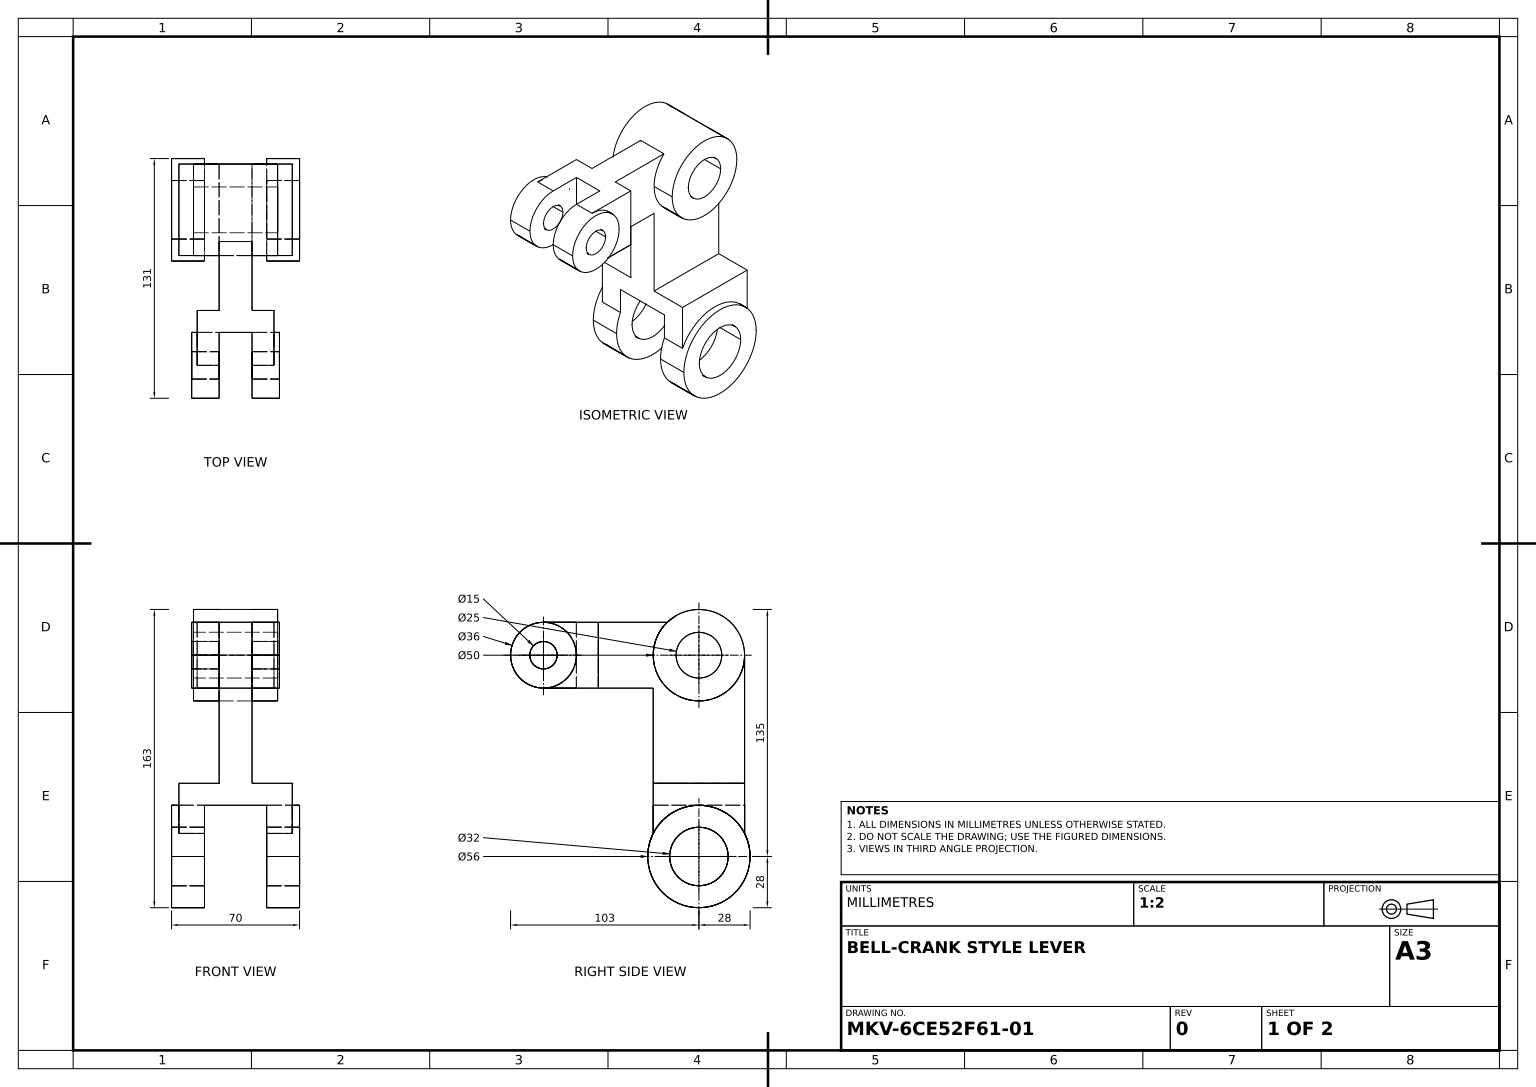
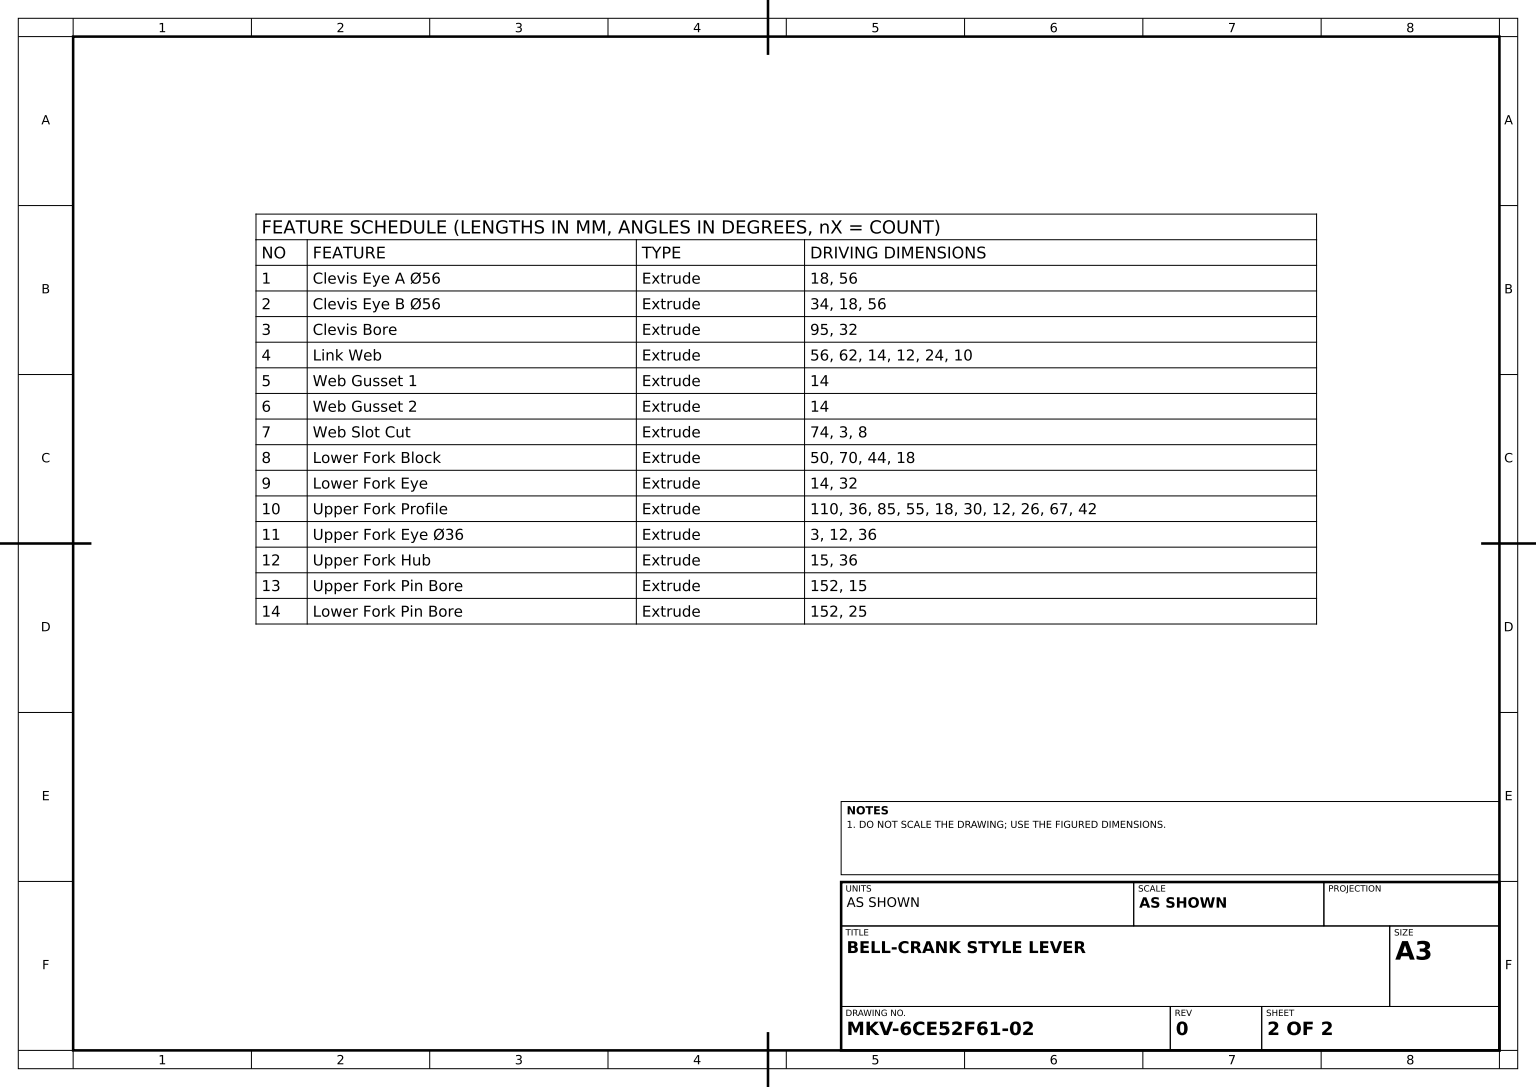
from build123d import *

# Parameters (mm, degrees)
CLEVIS_EYE_A_SKETCH_R        = 28
CLEVIS_EYE_A_56_DEPTH        = 18
CLEVIS_EYE_B_SKETCH_R        = 28
CLEVIS_EYE_B_56_DEPTH        = 18
CLEVIS_BORE_SKETCH_R         = 16
CLEVIS_BORE_DEPTH            = 95
LINK_WEB_DEPTH               = 28
WEB_GUSSET_1_DEPTH           = 14
WEB_START                    = -14
WEB_GUSSET_2_DEPTH           = 14
WEB_SLOT_CUT_DEPTH           = 74
LOWER_FORK_BLOCK_SKETCH_W    = 18
LOWER_FORK_BLOCK_SKETCH_H    = 70
LOWER_FORK_BLOCK_DEPTH       = 50
LOWER_FORK_EYE_DEPTH         = 14
LOWER_FORK_EYE_DEPTH_BACK    = 32
LOWER_FORK_EYE_SKETCH_R      = 25
UPPER_FORK_PROFILE_DEPTH     = 18
UPPER_FORK_EYE_36_DEPTH      = 3
UPPER_FORK_EYE_36_DEPTH_BACK = 12
UPPER_FORK_EYE_SKETCH_36_R   = 18
UPPER_FORK_HUB_SKETCH_R      = 18
UPPER_FORK_HUB_DEPTH         = 15
UPPER_FORK_PIN_BORE_SKETCH_R = 7.5
UPPER_FORK_PIN_BORE_DEPTH    = 152
LOWER_FORK_PIN_BORE_SKETCH_R = 12.5
LOWER_FORK_PIN_BORE_DEPTH    = 152


with BuildPart() as part:
    # Clevis Eye A Sketch → Clevis Eye A Ø56 (new body)
    with BuildSketch(Plane(origin=(0, 0, 0), x_dir=(0, 0, -1), z_dir=(1, 0, 0))):
        Circle(CLEVIS_EYE_A_SKETCH_R)
    extrude(amount=-CLEVIS_EYE_A_56_DEPTH)


with BuildPart() as body_2:
    # Clevis Eye B Sketch → Clevis Eye B Ø56 (new body)
    with BuildSketch(Plane.ZY.offset(52)):
        with Locations(Location((0, 0, 0), (0, 0, 180))):
            Circle(CLEVIS_EYE_B_SKETCH_R)
    extrude(amount=CLEVIS_EYE_B_56_DEPTH)


with BuildPart() as clevis_bore_tool:
    # Clevis Bore Sketch → Clevis Bore (new body)
    with BuildSketch(Plane(origin=(0, 0, 0), x_dir=(0, 0, -1), z_dir=(1, 0, 0))):
        Circle(CLEVIS_BORE_SKETCH_R)
    extrude(amount=-CLEVIS_BORE_DEPTH)


with BuildPart() as part_1:
    add(part.part)

    # Clevis Bore: cut by clevis_bore_tool
    add(clevis_bore_tool.part, mode=Mode.SUBTRACT)



with BuildPart() as body_2_1:
    add(body_2.part)

    # Clevis Bore: cut by clevis_bore_tool
    add(clevis_bore_tool.part, mode=Mode.SUBTRACT)


with BuildPart() as part_2:
    add(part_1.part)

    add(body_2_1.part)  # Link Web merges body 2
    # Link Web Sketch → Link Web (add, symmetric)
    with BuildSketch(Plane.XY):
        Polygon((-66, 40), (-66, 16), (-52, 16), (-52, 26), (-52, 28), (-18, 28), (-18, 26), (-18, 16), (-4, 16), (-4, 40), align=None)
    extrude(amount=LINK_WEB_DEPTH, both=True)

    # Web Gusset 1 Sketch → Web Gusset 1 (add)
    with BuildSketch(Plane(origin=(-4, 0, 0), x_dir=(0, 0, -1), z_dir=(1, 0, 0))):
        with BuildLine():
            Line((-28, 16), (-28, 0))
            ThreePointArc((-28, 0), (-26.71508, 8.384777), (-22.978251, 16))
            Line((-22.978251, 16), (-28, 16))
        make_face()
        with BuildLine():
            Line((28, 16), (28, 0))
            ThreePointArc((28, 0), (26.71508, 8.384777), (22.978251, 16))
            Line((22.978251, 16), (28, 16))
        make_face()
    extrude(amount=-WEB_GUSSET_1_DEPTH)

    # Web Gusset 2 Sketch → Web Gusset 2 (add)
    with BuildSketch(Plane.ZY.offset(66).offset(WEB_START)):
        with BuildLine():
            Line((28, 16), (28, 0))
            ThreePointArc((28, 0), (26.71508, 8.384777), (22.978251, 16))
            Line((22.978251, 16), (28, 16))
        make_face()
        with BuildLine():
            Line((-28, 0), (-28, 16))
            Line((-28, 16), (-22.978251, 16))
            ThreePointArc((-22.978251, 16), (-26.71508, 8.384777), (-28, 0))
        make_face()
    extrude(amount=WEB_GUSSET_2_DEPTH)

    # Web Slot Sketch → Web Slot Cut (cut)
    with BuildSketch(Plane(origin=(-4, 0, 0), x_dir=(0, 0, -1), z_dir=(1, 0, 0))):
        with BuildLine():
            Line((-25, 12.60952), (-25, 40))
            Line((-25, 40), (-28, 40))
            Line((-28, 40), (-28, 0))
            ThreePointArc((-28, 0), (-27.239677, 6.480741), (-25, 12.60952))
        make_face()
        with BuildLine():
            Line((28, 40), (25, 40))
            Line((25, 40), (25, 12.60952))
            ThreePointArc((25, 12.60952), (27.239677, 6.480741), (28, 0))
            Line((28, 0), (28, 40))
        make_face()
    extrude(amount=-WEB_SLOT_CUT_DEPTH, mode=Mode.SUBTRACT)

    # Lower Fork Block Sketch → Lower Fork Block (add)
    with BuildSketch(Plane.XY.offset(25)):
        with Locations((-35, 75)):
            Rectangle(LOWER_FORK_BLOCK_SKETCH_W, LOWER_FORK_BLOCK_SKETCH_H)
    extrude(amount=-LOWER_FORK_BLOCK_DEPTH)

    # Lower Fork Eye Sketch → Lower Fork Eye (add, two sides: drawn at the far end of the back side and taken through both)
    with BuildSketch(Plane.ZY.offset(44).offset(-LOWER_FORK_EYE_DEPTH_BACK)):
        with Locations((0, 110)):
            Circle(LOWER_FORK_EYE_SKETCH_R)
    extrude(amount=LOWER_FORK_EYE_DEPTH + LOWER_FORK_EYE_DEPTH_BACK)

    # Upper Fork Profile Sketch → Upper Fork Profile (add, symmetric)
    with BuildSketch(Plane(origin=(0, 110, 0), x_dir=(1, 0, 0), z_dir=(0, 1, 0))):
        Polygon((-26, -55), (-14, -55), (-14, -85), (-26, -85), (-26, -67), (-44, -67), (-44, -85), (-56, -85), (-56, -55), (-44, -55), (-44, 0), (-26, 0), align=None)
    extrude(amount=UPPER_FORK_PROFILE_DEPTH, both=True)

    # Upper Fork Eye Sketch Ø36 → Upper Fork Eye Ø36 (add, two sides: drawn at the far end of the back side and taken through both)
    with BuildSketch(Plane(origin=(-14, 0, 0), x_dir=(0, 0, -1), z_dir=(1, 0, 0)).offset(-UPPER_FORK_EYE_36_DEPTH_BACK)):
        with Locations((-85, 110)):
            Circle(UPPER_FORK_EYE_SKETCH_36_R)
    extrude(amount=UPPER_FORK_EYE_36_DEPTH + UPPER_FORK_EYE_36_DEPTH_BACK)

    # Upper Fork Hub Sketch → Upper Fork Hub (add)
    with BuildSketch(Plane(origin=(-44, 0, 0), x_dir=(0, 0, -1), z_dir=(1, 0, 0))):
        with Locations((-85, 110)):
            Circle(UPPER_FORK_HUB_SKETCH_R)
    extrude(amount=-UPPER_FORK_HUB_DEPTH)

    # Upper Fork Pin Bore Sketch → Upper Fork Pin Bore (cut)
    with BuildSketch(Plane(origin=(-11, 0, 0), x_dir=(0, 0, -1), z_dir=(1, 0, 0))):
        with Locations((-85, 110)):
            Circle(UPPER_FORK_PIN_BORE_SKETCH_R)
    extrude(amount=-UPPER_FORK_PIN_BORE_DEPTH, mode=Mode.SUBTRACT)

    # Lower Fork Pin Bore Sketch → Lower Fork Pin Bore (cut)
    with BuildSketch(Plane(origin=(-12, 0, 0), x_dir=(0, 0, -1), z_dir=(1, 0, 0))):
        with Locations((0, 110)):
            Circle(LOWER_FORK_PIN_BORE_SKETCH_R)
    extrude(amount=-LOWER_FORK_PIN_BORE_DEPTH, mode=Mode.SUBTRACT)


solid = part_2.part
